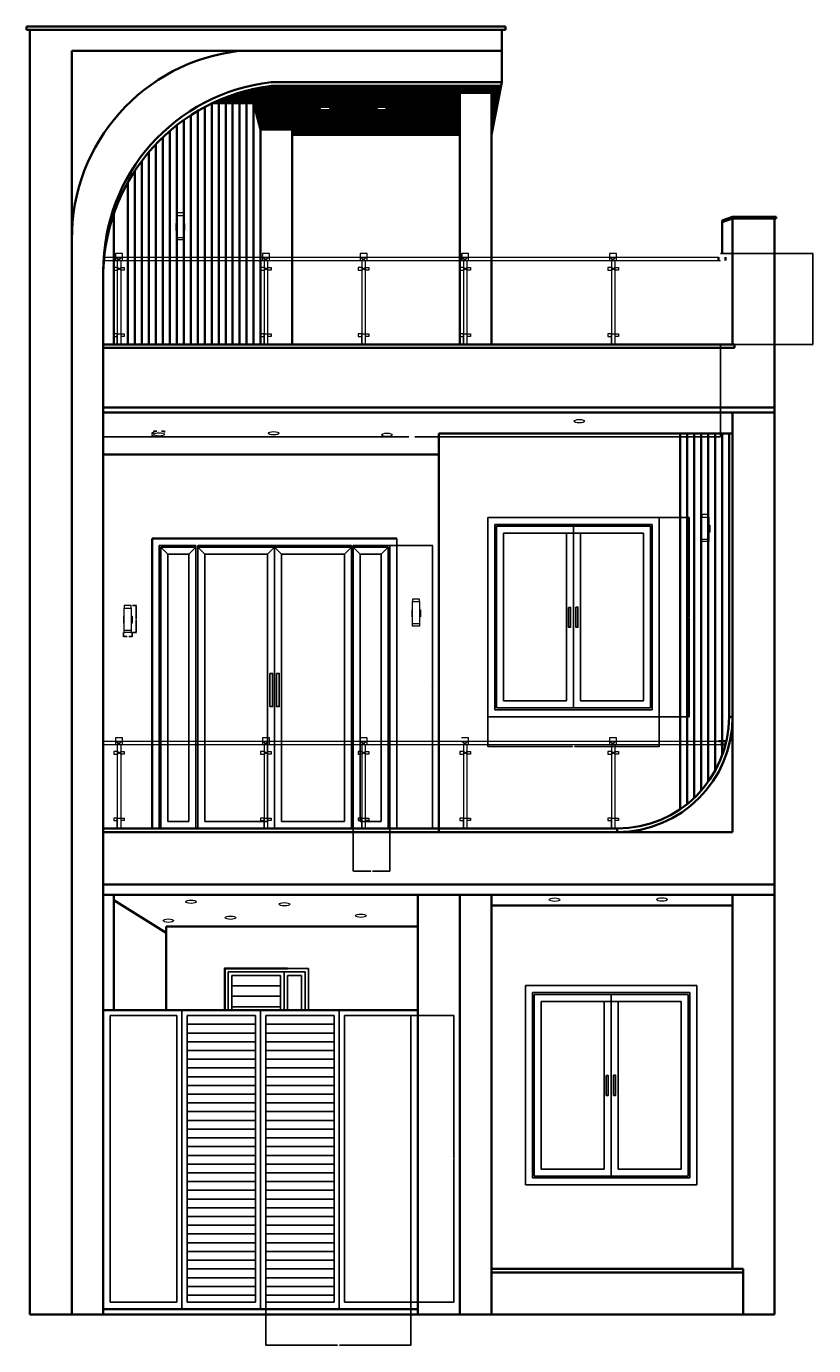
# Model space of a CAD drawing. Units: inches. Extents: x 2700 to 3150, y 1021 to 1776.
import ezdxf

# ---------------------------------------------------------------- set-up
doc = ezdxf.new("R2010")
doc.units = ezdxf.units.IN
doc.header["$MEASUREMENT"] = 0
for name, color, linetype, lineweight in [('A-ANNO-DIMS', 2, 'Continuous', 18), ('A-DOOR', 3, 'Continuous', 25), ('A-ELEV', 7, 'Continuous', 35), ('A-ELEV-CONS', 8, 'Continuous', 13), ('A-FLOR-HRAL', 6, 'Continuous', 18), ('A-GLAZ', 4, 'Continuous', 25), ('E-LITE', 2, 'Continuous', 18)]:
    doc.layers.add(name, color=color, linetype=linetype, lineweight=lineweight)
doc.styles.get("Standard").update_dxf_attribs({"font": 'arial.ttf'})
doc.dimstyles.get("Standard").update_dxf_attribs({"dimtxt": 0.18, "dimasz": 0.18, "dimexe": 0.18, "dimexo": 0.0625, "dimgap": 0.09, "dimtad": 0, "dimtih": 1, "dimtoh": 1, "dimdec": 1, "dimzin": 0, "dimdsep": 46, "dimlunit": 3, "dimtxsty": 'Standard', "dimcen": 0.09, "dimadec": 0, "dimazin": 0, "dimtfac": 1, "dimtdec": 1, "dimtofl": 0, "dimtmove": 0, "dimatfit": 3, "dimfxl": 1, "dimtolj": 1, "dimtzin": 0, "dimarcsym": 0})

# ---------------------------------------------------------------- blocks, each defined once
blk = doc.blocks.new('g')
for p, q in [((2754.61, 1646.14), (2750.61, 1646.14)), ((2750.61, 1646.14), (2750.61, 1642.14)), ((2754.61, 1642.14), (2754.61, 1646.14)), ((2838.61, 1646.14), (2834.61, 1646.14)), ((2834.61, 1646.14), (2834.61, 1642.14)), ((2838.61, 1642.14), (2838.61, 1646.14)), ((2894.49, 1646.14), (2890.49, 1646.14)), ((2890.49, 1646.14), (2890.49, 1642.14)), ((2894.49, 1642.14), (2894.49, 1646.14)), ((2952.61, 1646.14), (2948.61, 1646.14)), ((2952.61, 1642.14), (2952.61, 1646.14)), ((3037.26, 1646.14), (3033.26, 1646.14)), ((3033.26, 1646.14), (3033.26, 1642.14)), ((3037.26, 1642.14), (3037.26, 1646.14)), ((2743.61, 1644.14), (3095.61, 1644.14)), ((2743.61, 1642.14), (3096.61, 1642.14)), ((2751.61, 1638.14), (2749.61, 1638.14)), ((2749.61, 1638.14), (2749.61, 1636.64)), ((2750.61, 1644.14), (2753.61, 1642.14)), ((2750.61, 1642.14), (2751.61, 1642.14)), ((2754.61, 1644.14), (2751.61, 1642.14)), ((2751.61, 1642.14), (2751.61, 1594.14)), ((2751.61, 1636.64), (2753.61, 1638.14)), ((2753.61, 1636.64), (2751.61, 1638.14)), ((2753.61, 1642.14), (2754.61, 1642.14)), ((2753.61, 1642.14), (2753.61, 1594.14)), ((2753.61, 1642.14), (2753.61, 1638.14)), ((2753.61, 1638.14), (2755.61, 1638.14)), ((2755.61, 1638.14), (2755.61, 1636.64)), ((2835.61, 1638.14), (2833.61, 1638.14)), ((2833.61, 1638.14), (2833.61, 1636.64)), ((2834.61, 1644.14), (2837.61, 1642.14)), ((2834.61, 1642.14), (2835.61, 1642.14)), ((2838.61, 1644.14), (2835.61, 1642.14)), ((2835.61, 1642.14), (2835.61, 1594.14)), ((2835.61, 1636.64), (2837.61, 1638.14)), ((2837.61, 1636.64), (2835.61, 1638.14)), ((2837.61, 1642.14), (2838.61, 1642.14)), ((2837.61, 1642.14), (2837.61, 1594.14)), ((2837.61, 1642.14), (2837.61, 1638.14)), ((2837.61, 1638.14), (2839.61, 1638.14)), ((2839.61, 1638.14), (2839.61, 1636.64)), ((2891.49, 1638.14), (2889.49, 1638.14)), ((2889.49, 1638.14), (2889.49, 1636.64)), ((2890.49, 1644.14), (2893.49, 1642.14)), ((2890.49, 1642.14), (2891.49, 1642.14)), ((2894.49, 1644.14), (2891.49, 1642.14)), ((2891.49, 1642.14), (2891.49, 1594.14)), ((2891.49, 1636.64), (2893.49, 1638.14)), ((2893.49, 1636.64), (2891.49, 1638.14)), ((2893.49, 1642.14), (2894.49, 1642.14)), ((2893.49, 1642.14), (2893.49, 1594.14)), ((2893.49, 1642.14), (2893.49, 1638.14)), ((2893.49, 1638.14), (2895.49, 1638.14)), ((2895.49, 1638.14), (2895.49, 1636.64)), ((2949.61, 1638.14), (2947.61, 1638.14)), ((2947.61, 1638.14), (2947.61, 1636.64)), ((2948.61, 1644.14), (2951.61, 1642.14)), ((2948.61, 1642.14), (2949.61, 1642.14)), ((2952.61, 1644.14), (2949.61, 1642.14)), ((2949.61, 1642.14), (2949.61, 1594.14)), ((2949.61, 1636.64), (2951.61, 1638.14)), ((2951.61, 1636.64), (2949.61, 1638.14)), ((2951.61, 1642.14), (2952.61, 1642.14)), ((2951.61, 1642.14), (2951.61, 1594.14)), ((2951.61, 1642.14), (2951.61, 1638.14)), ((2951.61, 1638.14), (2953.61, 1638.14)), ((2953.61, 1638.14), (2953.61, 1636.64)), ((3034.26, 1638.14), (3032.26, 1638.14)), ((3032.26, 1638.14), (3032.26, 1636.64)), ((3033.26, 1644.14), (3036.26, 1642.14)), ((3033.26, 1642.14), (3034.26, 1642.14)), ((3037.26, 1644.14), (3034.26, 1642.14)), ((3034.26, 1642.14), (3034.26, 1594.14)), ((3034.26, 1636.64), (3036.26, 1638.14)), ((3036.26, 1636.64), (3034.26, 1638.14)), ((3036.26, 1642.14), (3037.26, 1642.14)), ((3036.26, 1642.14), (3036.26, 1594.14)), ((3036.26, 1642.14), (3036.26, 1638.14)), ((3036.26, 1638.14), (3038.26, 1638.14)), ((3038.26, 1638.14), (3038.26, 1636.64)), ((2749.61, 1636.64), (2751.61, 1636.64)), ((2755.61, 1636.64), (2753.61, 1636.64)), ((2833.61, 1636.64), (2835.61, 1636.64)), ((2839.61, 1636.64), (2837.61, 1636.64)), ((2889.49, 1636.64), (2891.49, 1636.64)), ((2895.49, 1636.64), (2893.49, 1636.64)), ((2947.61, 1636.64), (2949.61, 1636.64)), ((2953.61, 1636.64), (2951.61, 1636.64)), ((3032.26, 1636.64), (3034.26, 1636.64)), ((3038.26, 1636.64), (3036.26, 1636.64)), ((2751.61, 1600.16), (2749.61, 1600.16)), ((2749.61, 1600.16), (2749.61, 1598.66)), ((2749.61, 1598.66), (2751.61, 1598.66)), ((2751.61, 1594.14), (2751.61, 1600.16)), ((2751.61, 1600.16), (2753.61, 1600.16)), ((2753.61, 1600.16), (2755.61, 1600.16)), ((2755.61, 1598.66), (2753.61, 1598.66)), ((2755.61, 1600.16), (2755.61, 1598.66)), ((2835.61, 1600.16), (2833.61, 1600.16)), ((2833.61, 1600.16), (2833.61, 1598.66)), ((2833.61, 1598.66), (2835.61, 1598.66)), ((2835.61, 1594.14), (2835.61, 1600.16)), ((2835.61, 1600.16), (2837.61, 1600.16)), ((2837.61, 1600.16), (2839.61, 1600.16)), ((2839.61, 1598.66), (2837.61, 1598.66)), ((2839.61, 1600.16), (2839.61, 1598.66)), ((2891.49, 1600.16), (2889.49, 1600.16)), ((2889.49, 1600.16), (2889.49, 1598.66)), ((2889.49, 1598.66), (2891.49, 1598.66)), ((2891.49, 1594.14), (2891.49, 1600.16)), ((2891.49, 1600.16), (2893.49, 1600.16)), ((2893.49, 1600.16), (2895.49, 1600.16)), ((2895.49, 1598.66), (2893.49, 1598.66)), ((2895.49, 1600.16), (2895.49, 1598.66)), ((2949.61, 1600.16), (2947.61, 1600.16)), ((2947.61, 1600.16), (2947.61, 1598.66)), ((2947.61, 1598.66), (2949.61, 1598.66)), ((2949.61, 1594.14), (2949.61, 1600.16)), ((2949.61, 1600.16), (2951.61, 1600.16)), ((2951.61, 1600.16), (2953.61, 1600.16)), ((2953.61, 1598.66), (2951.61, 1598.66)), ((2953.61, 1600.16), (2953.61, 1598.66)), ((3034.26, 1600.16), (3032.26, 1600.16)), ((3032.26, 1600.16), (3032.26, 1598.66)), ((3032.26, 1598.66), (3034.26, 1598.66)), ((3034.26, 1594.14), (3034.26, 1600.16)), ((3034.26, 1600.16), (3036.26, 1600.16)), ((3036.26, 1600.16), (3038.26, 1600.16)), ((3038.26, 1598.66), (3036.26, 1598.66)), ((3038.26, 1600.16), (3038.26, 1598.66))]:
    blk.add_line(p, q)
blk = doc.blocks.new('l')
for p, q in [((3090.07, 1496.8), (3086.07, 1496.8)), ((3086.07, 1496.8), (3086.07, 1495.38)), ((3086.07, 1495.38), (3090.07, 1495.38)), ((3086.07, 1481.35), (3086.07, 1495.38)), ((3090.07, 1495.38), (3090.07, 1496.8)), ((3090.07, 1495.38), (3090.07, 1481.35)), ((3086.07, 1490.73), (3085.61, 1490.73)), ((3085.61, 1490.73), (3085.61, 1486.73)), ((3090.07, 1490.73), (3090.61, 1490.73)), ((3090.61, 1490.73), (3090.61, 1486.73)), ((3085.61, 1486.73), (3086.07, 1486.73)), ((3086.07, 1482.78), (3090.07, 1482.78)), ((3090.07, 1481.35), (3086.07, 1481.35)), ((3090.61, 1486.73), (3090.07, 1486.73))]:
    blk.add_line(p, q)
blk = doc.blocks.new('WIN-DOUBLE')
for p, q in [((2963.61, 1495.14), (2963.61, 1381.14)), ((2963.61, 1495.14), (3061.61, 1495.14)), ((3061.61, 1495.14), (3061.61, 1381.14)), ((2967.61, 1491.14), (2967.61, 1385.14)), ((2967.61, 1491.14), (3057.61, 1491.14)), ((2968.61, 1490.14), (2968.61, 1386.14)), ((2968.61, 1490.14), (3056.61, 1490.14)), ((3012.61, 1490.14), (3012.61, 1386.14)), ((3056.61, 1490.14), (3056.61, 1386.14)), ((3057.61, 1491.14), (3057.61, 1385.14)), ((2972.61, 1486.14), (3052.61, 1486.14)), ((2972.61, 1486.14), (2972.61, 1390.14)), ((3008.61, 1486.14), (3008.61, 1390.14)), ((3016.61, 1486.14), (3016.61, 1390.14)), ((3052.61, 1486.14), (3052.61, 1390.14)), ((2972.61, 1390.14), (3008.61, 1390.14)), ((3016.61, 1390.14), (3052.61, 1390.14)), ((2967.61, 1385.14), (3057.61, 1385.14)), ((2968.61, 1386.14), (3056.61, 1386.14)), ((2963.61, 1381.14), (3061.61, 1381.14))]:
    blk.add_line(p, q)
for points in [[(3009.78, 1443.68), (3010.92, 1443.68), (3010.92, 1432.35), (3009.78, 1432.35)], [(3013.96, 1443.85), (3015.09, 1443.85), (3015.09, 1432.33), (3013.96, 1432.33)]]:
    blk.add_lwpolyline(points, close=True)
blk = doc.blocks.new('DOOR-SIDELIGHT')
for p, q in [((2886.61, 1317.14), (2886.61, 1479.14)), ((2886.61, 1479.14), (2907.61, 1479.14)), ((2886.61, 1478.14), (2906.61, 1478.14)), ((2890.61, 1474.14), (2886.61, 1478.14)), ((2890.61, 1321.14), (2890.61, 1474.14)), ((2890.61, 1474.14), (2902.61, 1474.14)), ((2902.61, 1474.14), (2906.61, 1478.14)), ((2902.61, 1321.14), (2902.61, 1474.14)), ((2906.61, 1317.14), (2906.61, 1478.14)), ((2907.61, 1317.14), (2907.61, 1479.14)), ((2890.61, 1321.14), (2902.61, 1321.14))]:
    blk.add_line(p, q)
blk = doc.blocks.new('GATE-SIDE-PANEL')
for p, q in [((2836.61, 1210.14), (2836.61, 1046.14)), ((2875.61, 1210.14), (2836.61, 1210.14)), ((2875.61, 1210.14), (2875.61, 1046.14)), ((2881.61, 1210.14), (2881.61, 1046.14)), ((2919.61, 1210.14), (2881.61, 1210.14)), ((2919.61, 1210.14), (2919.61, 1046.14)), ((2836.61, 1046.14), (2875.61, 1046.14)), ((2881.61, 1046.14), (2919.61, 1046.14))]:
    blk.add_line(p, q)
blk = doc.blocks.new('LIGHT-COVE')
blk.add_ellipse((2870.52, 1729.14), major_axis=(-3.07, 0), ratio=0.316207)
blk = doc.blocks.new('*D7')
at = {"layer": 'A-ANNO-DIMS', "color": 0, "lineweight": -2, "transparency": 16777216}
for p, q in [((3061.67, 1495.14), (3078.89, 1495.14)), ((3078.71, 1494.96), (3078.71, 1438.32)), ((3078.71, 1381.32), (3078.71, 1437.96)), ((3061.67, 1381.14), (3078.89, 1381.14))]:
    blk.add_line(p, q, dxfattribs=at)
at = {"layer": 'A-ANNO-DIMS', "color": 0, "transparency": 16777216}
for points in [[(3078.68, 1494.96), (3078.74, 1494.96), (3078.71, 1495.14)], [(3078.68, 1381.32), (3078.74, 1381.32), (3078.71, 1381.14)]]:
    blk.add_solid(points, dxfattribs=at)
at = {"layer": 'Defpoints', "color": 0, "transparency": 16777216}
for p in [(3061.61, 1495.14), (3078.71, 1495.14), (3061.61, 1381.14)]:
    blk.add_point(p, dxfattribs=at)
at = {"layer": 'A-ANNO-DIMS', "color": 0, "transparency": 16777216, "insert": (3078.71, 1438.14), "char_height": 0.18, "attachment_point": 5}
blk.add_mtext('\\A1;WINDOW 114 TYP.', dxfattribs=at)
blk = doc.blocks.new('*D8')
at = {"layer": 'A-ANNO-DIMS', "color": 0, "lineweight": -2, "transparency": 16777216}
for p, q in [((2963.61, 1381.08), (2963.61, 1363.86)), ((3061.61, 1381.08), (3061.61, 1363.86)), ((2963.79, 1364.04), (3012.08, 1364.04)), ((3061.43, 1364.04), (3013.14, 1364.04))]:
    blk.add_line(p, q, dxfattribs=at)
at = {"layer": 'A-ANNO-DIMS', "color": 0, "transparency": 16777216}
for points in [[(2963.79, 1364.07), (2963.79, 1364.01), (2963.61, 1364.04)], [(3061.43, 1364.07), (3061.43, 1364.01), (3061.61, 1364.04)]]:
    blk.add_solid(points, dxfattribs=at)
at = {"layer": 'Defpoints', "color": 0, "transparency": 16777216}
for p in [(2963.61, 1381.14), (3061.61, 1381.14), (3061.61, 1364.04)]:
    blk.add_point(p, dxfattribs=at)
at = {"layer": 'A-ANNO-DIMS', "color": 0, "transparency": 16777216, "insert": (3012.61, 1364.04), "char_height": 0.18, "attachment_point": 5}
blk.add_mtext('\\A1;98 TYP.', dxfattribs=at)
blk = doc.blocks.new('*D9')
at = {"layer": 'A-ANNO-DIMS', "color": 0, "lineweight": -2, "transparency": 16777216}
for p, q in [((2907.67, 1479.14), (2932.09, 1479.14)), ((2931.91, 1478.96), (2931.91, 1398.32)), ((2931.91, 1317.32), (2931.91, 1397.96)), ((2907.67, 1317.14), (2932.09, 1317.14))]:
    blk.add_line(p, q, dxfattribs=at)
at = {"layer": 'A-ANNO-DIMS', "color": 0, "transparency": 16777216}
for points in [[(2931.88, 1478.96), (2931.94, 1478.96), (2931.91, 1479.14)], [(2931.88, 1317.32), (2931.94, 1317.32), (2931.91, 1317.14)]]:
    blk.add_solid(points, dxfattribs=at)
at = {"layer": 'Defpoints', "color": 0, "transparency": 16777216}
for p in [(2907.61, 1479.14), (2931.91, 1479.14), (2907.61, 1317.14)]:
    blk.add_point(p, dxfattribs=at)
at = {"layer": 'A-ANNO-DIMS', "color": 0, "transparency": 16777216, "insert": (2931.91, 1398.14), "char_height": 0.18, "attachment_point": 5}
blk.add_mtext('\\A1;DOOR SIDELIGHT 162 TYP.', dxfattribs=at)
blk = doc.blocks.new('*D10')
at = {"layer": 'A-ANNO-DIMS', "color": 0, "lineweight": -2, "transparency": 16777216}
for p, q in [((2886.61, 1317.08), (2886.61, 1292.66)), ((2907.61, 1317.08), (2907.61, 1292.66)), ((2886.79, 1292.84), (2896.58, 1292.84)), ((2907.43, 1292.84), (2897.64, 1292.84))]:
    blk.add_line(p, q, dxfattribs=at)
at = {"layer": 'A-ANNO-DIMS', "color": 0, "transparency": 16777216}
for points in [[(2886.79, 1292.87), (2886.79, 1292.81), (2886.61, 1292.84)], [(2907.43, 1292.87), (2907.43, 1292.81), (2907.61, 1292.84)]]:
    blk.add_solid(points, dxfattribs=at)
at = {"layer": 'Defpoints', "color": 0, "transparency": 16777216}
for p in [(2886.61, 1317.14), (2907.61, 1317.14), (2907.61, 1292.84)]:
    blk.add_point(p, dxfattribs=at)
at = {"layer": 'A-ANNO-DIMS', "color": 0, "transparency": 16777216, "insert": (2897.11, 1292.84), "char_height": 0.18, "attachment_point": 5}
blk.add_mtext('\\A1;21 TYP.', dxfattribs=at)
blk = doc.blocks.new('*D11')
at = {"layer": 'A-ANNO-DIMS', "color": 0, "lineweight": -2, "transparency": 16777216}
for p, q in [((2919.67, 1210.14), (2944.39, 1210.14)), ((2944.21, 1209.96), (2944.21, 1128.32)), ((2944.21, 1046.32), (2944.21, 1127.96)), ((2919.67, 1046.14), (2944.39, 1046.14))]:
    blk.add_line(p, q, dxfattribs=at)
at = {"layer": 'A-ANNO-DIMS', "color": 0, "transparency": 16777216}
for points in [[(2944.18, 1209.96), (2944.24, 1209.96), (2944.21, 1210.14)], [(2944.18, 1046.32), (2944.24, 1046.32), (2944.21, 1046.14)]]:
    blk.add_solid(points, dxfattribs=at)
at = {"layer": 'Defpoints', "color": 0, "transparency": 16777216}
for p in [(2919.61, 1210.14), (2944.21, 1210.14), (2919.61, 1046.14)]:
    blk.add_point(p, dxfattribs=at)
at = {"layer": 'A-ANNO-DIMS', "color": 0, "transparency": 16777216, "insert": (2944.21, 1128.14), "char_height": 0.18, "attachment_point": 5}
blk.add_mtext('\\A1;GATE SIDE PANEL 164 TYP.', dxfattribs=at)
blk = doc.blocks.new('*D12')
at = {"layer": 'A-ANNO-DIMS', "color": 0, "lineweight": -2, "transparency": 16777216}
for p, q in [((2836.61, 1046.08), (2836.61, 1021.36)), ((2919.61, 1046.08), (2919.61, 1021.36)), ((2836.79, 1021.54), (2877.58, 1021.54)), ((2919.43, 1021.54), (2878.64, 1021.54))]:
    blk.add_line(p, q, dxfattribs=at)
at = {"layer": 'A-ANNO-DIMS', "color": 0, "transparency": 16777216}
for points in [[(2836.79, 1021.57), (2836.79, 1021.51), (2836.61, 1021.54)], [(2919.43, 1021.57), (2919.43, 1021.51), (2919.61, 1021.54)]]:
    blk.add_solid(points, dxfattribs=at)
at = {"layer": 'Defpoints', "color": 0, "transparency": 16777216}
for p in [(2836.61, 1046.14), (2919.61, 1046.14), (2919.61, 1021.54)]:
    blk.add_point(p, dxfattribs=at)
at = {"layer": 'A-ANNO-DIMS', "color": 0, "transparency": 16777216, "insert": (2878.11, 1021.54), "char_height": 0.18, "attachment_point": 5}
blk.add_mtext('\\A1;83 TYP.', dxfattribs=at)
blk = doc.blocks.new('*D13')
at = {"layer": 'A-ANNO-DIMS', "color": 0, "lineweight": -2, "transparency": 16777216}
for p, q in [((2743.61, 1594.08), (2743.61, 1541.01)), ((3096.61, 1594.08), (3096.61, 1541.01)), ((2743.79, 1541.19), (2918.34, 1541.19)), ((3096.43, 1541.19), (2921.88, 1541.19))]:
    blk.add_line(p, q, dxfattribs=at)
at = {"layer": 'A-ANNO-DIMS', "color": 0, "transparency": 16777216}
for points in [[(2743.79, 1541.22), (2743.79, 1541.16), (2743.61, 1541.19)], [(3096.43, 1541.22), (3096.43, 1541.16), (3096.61, 1541.19)]]:
    blk.add_solid(points, dxfattribs=at)
at = {"layer": 'Defpoints', "color": 0, "transparency": 16777216}
for p in [(2743.61, 1594.14), (3096.61, 1594.14), (3096.61, 1541.19)]:
    blk.add_point(p, dxfattribs=at)
at = {"layer": 'A-ANNO-DIMS', "color": 0, "transparency": 16777216, "insert": (2920.11, 1541.19), "char_height": 0.18, "attachment_point": 5}
blk.add_mtext('\\A1;BALCONY RAILING 353 TYP.', dxfattribs=at)
blk = doc.blocks.new('*D14')
at = {"layer": 'A-ANNO-DIMS', "color": 0, "lineweight": -2, "transparency": 16777216}
for p, q in [((3096.67, 1646.14), (3149.74, 1646.14)), ((3149.56, 1645.96), (3149.56, 1620.32)), ((3149.56, 1594.32), (3149.56, 1619.96)), ((3096.67, 1594.14), (3149.74, 1594.14))]:
    blk.add_line(p, q, dxfattribs=at)
at = {"layer": 'A-ANNO-DIMS', "color": 0, "transparency": 16777216}
for points in [[(3149.53, 1645.96), (3149.59, 1645.96), (3149.56, 1646.14)], [(3149.53, 1594.32), (3149.59, 1594.32), (3149.56, 1594.14)]]:
    blk.add_solid(points, dxfattribs=at)
at = {"layer": 'Defpoints', "color": 0, "transparency": 16777216}
for p in [(3096.61, 1646.14), (3149.56, 1646.14), (3096.61, 1594.14)]:
    blk.add_point(p, dxfattribs=at)
at = {"layer": 'A-ANNO-DIMS', "color": 0, "transparency": 16777216, "insert": (3149.56, 1620.14), "char_height": 0.18, "attachment_point": 5}
blk.add_mtext('\\A1;52 TYP.', dxfattribs=at)
blk = doc.blocks.new('*D15')
at = {"layer": 'A-ANNO-DIMS', "color": 0, "lineweight": -2, "transparency": 16777216}
for p, q in [((2772.49, 1543.72), (2772.49, 1544.75)), ((2772.67, 1544.57), (2774.3, 1544.57)), ((2778.45, 1544.57), (2776.81, 1544.57)), ((2778.63, 1543.72), (2778.63, 1544.75))]:
    blk.add_line(p, q, dxfattribs=at)
at = {"layer": 'A-ANNO-DIMS', "color": 0, "transparency": 16777216}
for points in [[(2772.67, 1544.6), (2772.67, 1544.54), (2772.49, 1544.57)], [(2778.45, 1544.6), (2778.45, 1544.54), (2778.63, 1544.57)]]:
    blk.add_solid(points, dxfattribs=at)
at = {"layer": 'Defpoints', "color": 0, "transparency": 16777216}
for p in [(2772.49, 1544.57), (2772.49, 1543.65), (2778.63, 1543.65)]:
    blk.add_point(p, dxfattribs=at)
at = {"layer": 'A-ANNO-DIMS', "color": 0, "transparency": 16777216, "insert": (2775.56, 1544.57), "char_height": 0.18, "attachment_point": 5}
blk.add_mtext('\\A1;DOWNLIGHT 6 TYP.', dxfattribs=at)
blk = doc.blocks.new('*D16')
at = {"layer": 'A-ANNO-DIMS', "color": 0, "lineweight": -2, "transparency": 16777216}
for p, q in [((2772.43, 1543.65), (2771.39, 1543.65)), ((2772.43, 1541.71), (2771.39, 1541.71)), ((2771.57, 1543.47), (2771.57, 1542.86)), ((2771.57, 1541.89), (2771.57, 1542.5))]:
    blk.add_line(p, q, dxfattribs=at)
at = {"layer": 'A-ANNO-DIMS', "color": 0, "transparency": 16777216}
for points in [[(2771.54, 1543.47), (2771.6, 1543.47), (2771.57, 1543.65)], [(2771.54, 1541.89), (2771.6, 1541.89), (2771.57, 1541.71)]]:
    blk.add_solid(points, dxfattribs=at)
at = {"layer": 'Defpoints', "color": 0, "transparency": 16777216}
for p in [(2771.57, 1541.71), (2772.49, 1543.65), (2772.49, 1541.71)]:
    blk.add_point(p, dxfattribs=at)
at = {"layer": 'A-ANNO-DIMS', "color": 0, "transparency": 16777216, "insert": (2771.57, 1542.68), "char_height": 0.18, "attachment_point": 5}
blk.add_mtext('\\A1;2 TYP.', dxfattribs=at)
blk = doc.blocks.new('*D17')
at = {"layer": 'A-ANNO-DIMS', "color": 0, "lineweight": -2, "transparency": 16777216}
for p, q in [((2760.23, 1444.73), (2762.66, 1444.73)), ((2762.48, 1444.55), (2762.48, 1437.19)), ((2762.48, 1429.47), (2762.48, 1436.83)), ((2760.23, 1429.29), (2762.66, 1429.29))]:
    blk.add_line(p, q, dxfattribs=at)
at = {"layer": 'A-ANNO-DIMS', "color": 0, "transparency": 16777216}
for points in [[(2762.45, 1444.55), (2762.51, 1444.55), (2762.48, 1444.73)], [(2762.45, 1429.47), (2762.51, 1429.47), (2762.48, 1429.29)]]:
    blk.add_solid(points, dxfattribs=at)
at = {"layer": 'Defpoints', "color": 0, "transparency": 16777216}
for p in [(2760.16, 1444.73), (2762.48, 1444.73), (2760.16, 1429.29)]:
    blk.add_point(p, dxfattribs=at)
at = {"layer": 'A-ANNO-DIMS', "color": 0, "transparency": 16777216, "insert": (2762.48, 1437.01), "char_height": 0.18, "attachment_point": 5}
blk.add_mtext('\\A1;WALL LIGHT 15 TYP.', dxfattribs=at)
blk = doc.blocks.new('*D18')
at = {"layer": 'A-ANNO-DIMS', "color": 0, "lineweight": -2, "transparency": 16777216}
for p, q in [((2755.16, 1429.23), (2755.16, 1426.79)), ((2755.34, 1426.97), (2757.2, 1426.97)), ((2759.98, 1426.97), (2758.12, 1426.97)), ((2760.16, 1429.23), (2760.16, 1426.79))]:
    blk.add_line(p, q, dxfattribs=at)
at = {"layer": 'A-ANNO-DIMS', "color": 0, "transparency": 16777216}
for points in [[(2755.34, 1427), (2755.34, 1426.94), (2755.16, 1426.97)], [(2759.98, 1427), (2759.98, 1426.94), (2760.16, 1426.97)]]:
    blk.add_solid(points, dxfattribs=at)
at = {"layer": 'Defpoints', "color": 0, "transparency": 16777216}
for p in [(2755.16, 1429.29), (2760.16, 1429.29), (2760.16, 1426.97)]:
    blk.add_point(p, dxfattribs=at)
at = {"layer": 'A-ANNO-DIMS', "color": 0, "transparency": 16777216, "insert": (2757.66, 1426.97), "char_height": 0.18, "attachment_point": 5}
blk.add_mtext('\\A1;5 TYP.', dxfattribs=at)

msp = doc.modelspace()

# ---------------------------------------------------------------- linework, layer by layer
at = {"layer": 'A-DOOR'}
for p, q in [((2911.61, 1317.14), (2911.61, 1483.14)), ((2797.61, 1317.14), (2797.61, 1479.14)), ((2797.61, 1479.14), (2885.61, 1479.14)), ((2797.61, 1478.14), (2885.61, 1478.14)), ((2801.61, 1474.14), (2797.61, 1478.14)), ((2801.61, 1321.14), (2801.61, 1474.14)), ((2801.61, 1474.14), (2837.61, 1474.14)), ((2841.61, 1478.14), (2837.61, 1474.14)), ((2837.61, 1321.14), (2837.61, 1474.14)), ((2841.61, 1317.14), (2841.61, 1478.14)), ((2845.61, 1474.14), (2841.61, 1478.14)), ((2845.61, 1321.14), (2845.61, 1474.14)), ((2845.61, 1474.14), (2881.61, 1474.14)), ((2881.61, 1474.14), (2885.61, 1478.14)), ((2881.61, 1321.14), (2881.61, 1474.14)), ((2885.61, 1317.14), (2885.61, 1479.14)), ((2801.61, 1321.14), (2837.61, 1321.14)), ((2845.61, 1321.14), (2881.61, 1321.14)), ((2788.61, 1213.14), (2788.61, 1042.14)), ((2833.61, 1213.14), (2833.61, 1042.14)), ((2878.61, 1213.14), (2878.61, 1042.14)), ((2830.61, 1205.14), (2791.61, 1205.14)), ((2875.61, 1205.14), (2836.61, 1205.14)), ((2830.61, 1200.14), (2791.61, 1200.14)), ((2830.61, 1195.14), (2791.61, 1195.14)), ((2875.61, 1200.14), (2836.61, 1200.14)), ((2875.61, 1195.14), (2836.61, 1195.14)), ((2830.61, 1190.14), (2791.61, 1190.14)), ((2875.61, 1190.14), (2836.61, 1190.14)), ((2830.61, 1185.14), (2791.61, 1185.14)), ((2830.61, 1180.14), (2791.61, 1180.14)), ((2875.61, 1185.14), (2836.61, 1185.14)), ((2875.61, 1180.14), (2836.61, 1180.14)), ((2830.61, 1175.14), (2791.61, 1175.14)), ((2830.61, 1170.14), (2791.61, 1170.14)), ((2875.61, 1175.14), (2836.61, 1175.14)), ((2875.61, 1170.14), (2836.61, 1170.14)), ((2830.61, 1165.14), (2791.61, 1165.14)), ((2875.61, 1165.14), (2836.61, 1165.14)), ((2830.61, 1160.14), (2791.61, 1160.14)), ((2830.61, 1155.14), (2791.61, 1155.14)), ((2875.61, 1160.14), (2836.61, 1160.14)), ((2875.61, 1155.14), (2836.61, 1155.14)), ((2830.61, 1150.14), (2791.61, 1150.14)), ((2875.61, 1150.14), (2836.61, 1150.14)), ((2830.61, 1145.14), (2791.61, 1145.14)), ((2830.61, 1140.14), (2791.61, 1140.14)), ((2875.61, 1145.14), (2836.61, 1145.14)), ((2875.61, 1140.14), (2836.61, 1140.14)), ((2830.61, 1135.14), (2791.61, 1135.14)), ((2875.61, 1135.14), (2836.61, 1135.14)), ((2830.61, 1130.14), (2791.61, 1130.14)), ((2830.61, 1125.14), (2791.61, 1125.14)), ((2875.61, 1130.14), (2836.61, 1130.14)), ((2875.61, 1125.14), (2836.61, 1125.14)), ((2830.61, 1120.14), (2791.61, 1120.14)), ((2875.61, 1120.14), (2836.61, 1120.14)), ((2830.61, 1115.14), (2791.61, 1115.14)), ((2830.61, 1110.14), (2791.61, 1110.14)), ((2875.61, 1115.14), (2836.61, 1115.14)), ((2875.61, 1110.14), (2836.61, 1110.14)), ((2830.61, 1105.14), (2791.61, 1105.14)), ((2875.61, 1105.14), (2836.61, 1105.14)), ((2830.61, 1100.14), (2791.61, 1100.14)), ((2830.61, 1095.14), (2791.61, 1095.14)), ((2875.61, 1100.14), (2836.61, 1100.14)), ((2875.61, 1095.14), (2836.61, 1095.14)), ((2830.61, 1090.14), (2791.61, 1090.14)), ((2875.61, 1090.14), (2836.61, 1090.14)), ((2830.61, 1085.14), (2791.61, 1085.14)), ((2830.61, 1080.14), (2791.61, 1080.14)), ((2875.61, 1085.14), (2836.61, 1085.14)), ((2875.61, 1080.14), (2836.61, 1080.14)), ((2830.61, 1075.14), (2791.61, 1075.14)), ((2875.61, 1075.14), (2836.61, 1075.14)), ((2830.61, 1070.14), (2791.61, 1070.14)), ((2830.61, 1065.14), (2791.61, 1065.14)), ((2875.61, 1070.14), (2836.61, 1070.14)), ((2875.61, 1065.14), (2836.61, 1065.14)), ((2830.61, 1060.14), (2791.61, 1060.14)), ((2875.61, 1060.14), (2836.61, 1060.14)), ((2830.61, 1055.14), (2791.61, 1055.14)), ((2830.61, 1050.14), (2791.61, 1050.14)), ((2875.61, 1055.14), (2836.61, 1055.14)), ((2875.61, 1050.14), (2836.61, 1050.14))]:
    msp.add_line(p, q, dxfattribs=at)
for points in [[(2838.88, 1405.9), (2840.47, 1405.9), (2840.47, 1386.9), (2838.88, 1386.9)], [(2842.67, 1405.9), (2844.26, 1405.9), (2844.26, 1386.9), (2842.67, 1386.9)]]:
    msp.add_lwpolyline(points, close=True, dxfattribs=at)
at = {"layer": 'A-ELEV'}
for p, q in [((2701.61, 1776.14), (2699.61, 1776.14)), ((2699.61, 1776.14), (2699.61, 1774.14)), ((2699.61, 1774.14), (2701.61, 1774.14)), ((2701.61, 1776.14), (2971.61, 1776.14)), ((2701.61, 1039.14), (2701.61, 1774.14)), ((2701.61, 1774.14), (2971.61, 1774.14)), ((2973.61, 1776.14), (2971.61, 1776.14)), ((2971.61, 1744.14), (2971.61, 1774.14)), ((2971.61, 1774.14), (2973.61, 1774.14)), ((2973.61, 1774.14), (2973.61, 1776.14)), ((2725.61, 1039.14), (2725.61, 1762.14)), ((2725.61, 1762.14), (2971.61, 1762.14)), ((2839.61, 1744.14), (2971.61, 1744.14)), ((2971.61, 1744.14), (2965.61, 1714.14)), ((2818.11, 1737.14), (2947.61, 1737.14)), ((2821.19, 1738.14), (2947.61, 1738.14)), ((2824.64, 1739.14), (2970.61, 1739.14)), ((2828.59, 1740.14), (2970.81, 1740.14)), ((2833.35, 1741.14), (2971.01, 1741.14)), ((2839.61, 1742.14), (2971.21, 1742.14)), ((2947.61, 1738.14), (2947.61, 1594.14)), ((2970.41, 1738.14), (2947.61, 1738.14)), ((2965.61, 1738.14), (2965.61, 1594.14)), ((2965.61, 1737.14), (2970.21, 1737.14)), ((2801.61, 1729.97), (2801.61, 1594.14)), ((2805.61, 1732.01), (2805.61, 1594.14)), ((2829.61, 1732.14), (2805.89, 1732.14)), ((2808.02, 1733.14), (2947.61, 1733.14)), ((2809.61, 1732.14), (2809.61, 1594.14)), ((2810.29, 1734.14), (2947.61, 1734.14)), ((2812.7, 1735.14), (2947.61, 1735.14)), ((2813.61, 1732.14), (2813.61, 1594.14)), ((2815.3, 1736.14), (2947.61, 1736.14)), ((2817.61, 1732.14), (2817.61, 1594.14)), ((2821.61, 1732.14), (2821.61, 1594.14)), ((2825.61, 1732.14), (2825.61, 1594.14)), ((2829.61, 1732.14), (2829.61, 1594.14)), ((2829.61, 1732.14), (2947.61, 1732.14)), ((2829.61, 1732.14), (2833.61, 1717.14)), ((2829.87, 1731.14), (2947.61, 1731.14)), ((2830.14, 1730.14), (2947.61, 1730.14)), ((2830.41, 1729.14), (2867.35, 1729.14)), ((2873.49, 1729.14), (2900.06, 1729.14)), ((2905.73, 1729.14), (2947.61, 1729.14)), ((2965.61, 1736.14), (2970.01, 1736.14)), ((2965.61, 1735.14), (2969.81, 1735.14)), ((2965.61, 1734.14), (2969.61, 1734.14)), ((2965.61, 1733.14), (2969.41, 1733.14)), ((2965.61, 1732.14), (2969.21, 1732.14)), ((2965.61, 1731.14), (2969.01, 1731.14)), ((2965.61, 1730.14), (2968.81, 1730.14)), ((2965.61, 1729.14), (2968.61, 1729.14)), ((2789.61, 1722.51), (2789.61, 1594.14)), ((2793.61, 1725.23), (2793.61, 1594.14)), ((2797.61, 1727.71), (2797.61, 1594.14)), ((2830.67, 1728.14), (2947.61, 1728.14)), ((2830.94, 1727.14), (2947.61, 1727.14)), ((2831.21, 1726.14), (2947.61, 1726.14)), ((2831.47, 1725.14), (2947.61, 1725.14)), ((2831.74, 1724.14), (2947.61, 1724.14)), ((2832.01, 1723.14), (2947.61, 1723.14)), ((2832.27, 1722.14), (2947.61, 1722.14)), ((2832.54, 1721.14), (2947.61, 1721.14)), ((2965.61, 1728.14), (2968.41, 1728.14)), ((2965.61, 1727.14), (2968.21, 1727.14)), ((2965.61, 1726.14), (2968.01, 1726.14)), ((2965.61, 1725.14), (2967.81, 1725.14)), ((2965.61, 1724.14), (2967.61, 1724.14)), ((2965.61, 1723.14), (2967.41, 1723.14)), ((2965.61, 1722.14), (2967.21, 1722.14)), ((2965.61, 1721.14), (2967.01, 1721.14)), ((2781.61, 1716.21), (2781.61, 1594.14)), ((2785.61, 1719.51), (2785.61, 1594.14)), ((2832.81, 1720.14), (2947.61, 1720.14)), ((2833.07, 1719.14), (2947.61, 1719.14)), ((2833.34, 1718.14), (2947.61, 1718.14)), ((2833.61, 1717.14), (2833.61, 1594.14)), ((2833.61, 1717.14), (2947.61, 1717.14)), ((2851.61, 1717.14), (2851.61, 1594.14)), ((2851.61, 1716.14), (2947.61, 1716.14)), ((2851.61, 1715.14), (2947.61, 1715.14)), ((2851.61, 1714.14), (2947.61, 1714.14)), ((2965.61, 1720.14), (2966.81, 1720.14)), ((2965.61, 1719.14), (2966.61, 1719.14)), ((2965.61, 1718.14), (2966.41, 1718.14)), ((2965.61, 1717.14), (2966.21, 1717.14)), ((2773.61, 1708.55), (2773.61, 1594.14)), ((2777.61, 1712.57), (2777.61, 1594.14)), ((2765.61, 1699.07), (2765.61, 1594.14)), ((2769.61, 1704.08), (2769.61, 1594.14)), ((2761.61, 1693.37), (2761.61, 1594.14)), ((2757.61, 1686.79), (2757.61, 1594.14)), ((2749.61, 1668.97), (2749.61, 1594.14)), ((3097.61, 1665.14), (3103.61, 1667.14)), ((3103.61, 1666.14), (3097.61, 1664.14)), ((3097.61, 1664.14), (3097.61, 1665.14)), ((3097.61, 1664.14), (3097.61, 1646.14)), ((3103.61, 1667.14), (3103.61, 1594.14)), ((3103.61, 1667.14), (3127.61, 1667.14)), ((3103.61, 1666.14), (3127.61, 1666.14)), ((3127.61, 1667.14), (3128.61, 1667.14)), ((3127.61, 1666.14), (3127.61, 1039.14)), ((3128.61, 1666.14), (3127.61, 1666.14)), ((3128.61, 1667.14), (3128.61, 1666.14)), ((2948.61, 1646.14), (2948.61, 1642.14)), ((3095.61, 1644.14), (3095.61, 1642.14)), ((3099.61, 1644.14), (3099.61, 1642.14)), ((2743.61, 1039.14), (2743.61, 1637.48)), ((2743.61, 1594.14), (3103.61, 1594.14)), ((3103.61, 1594.14), (3104.61, 1594.14)), ((3104.61, 1594.14), (3104.61, 1592.14)), ((2743.61, 1592.14), (3103.61, 1592.14)), ((3104.61, 1592.14), (3103.61, 1592.14)), ((2743.61, 1558.14), (3127.61, 1558.14)), ((2743.61, 1555.14), (3127.61, 1555.14)), ((3103.61, 1555.14), (3103.61, 1315.14)), ((2935.61, 1315.14), (2935.61, 1543.14)), ((2935.61, 1543.14), (3103.61, 1543.14)), ((3073.61, 1543.14), (3073.61, 1328.23)), ((3077.61, 1543.14), (3077.61, 1331.18)), ((3081.61, 1543.14), (3081.61, 1334.66)), ((3085.61, 1543.14), (3085.61, 1338.81)), ((3089.61, 1543.14), (3089.61, 1343.83)), ((3093.61, 1543.14), (3093.61, 1350.16)), ((3097.61, 1543.14), (3097.61, 1358.87)), ((3103.61, 1543.14), (3101.61, 1543.14)), ((3101.61, 1543.14), (3101.61, 1381.14)), ((2743.61, 1531.14), (2935.61, 1531.14)), ((2771.61, 1317.14), (2771.61, 1483.14)), ((2771.61, 1483.14), (2911.61, 1483.14)), ((3103.61, 1381.14), (3101.61, 1381.14)), ((3095.61, 1367.14), (3100.05, 1367.1)), ((3096.61, 1365.14), (3099.58, 1365.15)), ((2743.61, 1317.14), (3037.61, 1317.14)), ((2743.61, 1315.14), (3103.61, 1315.14)), ((3037.61, 1317.14), (3037.61, 1315.14)), ((2743.61, 1285.14), (3127.61, 1285.14)), ((2743.61, 1279.14), (3127.61, 1279.14)), ((2749.61, 1279.14), (2749.61, 1213.14)), ((2749.61, 1276.13), (2779.61, 1257.45)), ((2923.61, 1279.14), (2923.61, 1039.14)), ((2947.61, 1279.14), (2947.61, 1039.14)), ((2947.61, 1279.14), (2947.61, 1039.14)), ((2965.61, 1279.14), (2965.61, 1039.14)), ((3103.61, 1279.14), (3103.61, 1065.14)), ((2965.61, 1273.14), (3103.61, 1273.14)), ((2923.61, 1261.14), (2779.61, 1261.14)), ((2779.61, 1261.14), (2779.61, 1213.14)), ((2923.61, 1213.14), (2743.61, 1213.14)), ((2965.61, 1065.14), (3109.61, 1065.14)), ((3109.61, 1065.14), (3109.61, 1039.14)), ((2965.61, 1063.14), (3109.61, 1063.14)), ((2743.61, 1042.14), (2923.61, 1042.14)), ((2701.61, 1039.14), (3127.61, 1039.14))]:
    msp.add_line(p, q, dxfattribs=at)
msp.add_lwpolyline([(2813.05, 1213.14), (2813.05, 1237.14), (2849.05, 1237.14)], dxfattribs=at)
for centre, radius, start, end in [((2833.61, 1654.81), 108, 96.37827, 180.35466), ((2851.61, 1636.81), 108, 96.37827, 180.35466), ((2853.58, 1633), 110.02, 97.17859, 178.35781), ((3037.61, 1381.14), 66, 270, 0), ((3037.61, 1381.14), 64, 270, 0)]:
    msp.add_arc(centre, radius, start, end, dxfattribs=at)
at = {"layer": 'A-ELEV-CONS'}
for p in [(2788.61, 1213.14), (2833.61, 1213.14), (2878.61, 1213.14)]:
    msp.add_point(p, dxfattribs=at)
at = {"layer": 'A-GLAZ'}
for p, q in [((2817.05, 1213.14), (2817.05, 1233.14)), ((2817.05, 1233.14), (2845.05, 1233.14)), ((2845.05, 1233.14), (2845.05, 1213.14)), ((2847.05, 1235.14), (2859.05, 1235.14)), ((2849.05, 1237.14), (2861.05, 1237.14)), ((2849.05, 1233.14), (2857.05, 1233.14)), ((2857.05, 1233.14), (2857.05, 1213.14)), ((2859.05, 1235.14), (2859.05, 1213.14)), ((2861.05, 1237.14), (2861.05, 1213.14)), ((2817.05, 1227.14), (2845.05, 1227.14)), ((2817.05, 1221.14), (2845.05, 1221.14)), ((2817.05, 1215.14), (2845.05, 1215.14))]:
    msp.add_line(p, q, dxfattribs=at)
for points in [[(2815.05, 1213.14), (2815.05, 1235.14), (2847.05, 1235.14), (2847.05, 1213.14)], [(2849.05, 1233.14), (2849.05, 1213.14)]]:
    msp.add_lwpolyline(points, dxfattribs=at)
at = {"layer": 'E-LITE'}
for p, q in [((2789.61, 1669.39), (2785.61, 1669.39)), ((2785.61, 1669.39), (2785.61, 1667.97)), ((2789.61, 1667.97), (2789.61, 1669.39)), ((2785.61, 1663.32), (2785.14, 1663.32)), ((2785.14, 1663.32), (2785.14, 1659.32)), ((2785.61, 1667.97), (2789.61, 1667.97)), ((2785.61, 1653.95), (2785.61, 1667.97)), ((2789.61, 1667.97), (2789.61, 1653.95)), ((2789.61, 1663.32), (2790.14, 1663.32)), ((2790.14, 1663.32), (2790.14, 1659.32)), ((2785.14, 1659.32), (2785.61, 1659.32)), ((2785.61, 1653.95), (2785.61, 1655.37)), ((2785.61, 1655.37), (2789.61, 1655.37)), ((2789.61, 1653.95), (2785.61, 1653.95)), ((2790.14, 1659.32), (2789.61, 1659.32)), ((2789.61, 1655.37), (2789.61, 1653.95))]:
    msp.add_line(p, q, dxfattribs=at)
msp.add_ellipse((2902.9, 1729.11), major_axis=(2.83, 0), ratio=0.342534, dxfattribs=at)

# ---------------------------------------------------------------- block references
at = {"layer": 'A-DOOR', "extrusion": (0, 0, -1), "zscale": -1}
msp.add_blockref('DOOR-SIDELIGHT', (-5683.22, 0), dxfattribs=at)
at = {"layer": 'A-DOOR'}
for name in ['DOOR-SIDELIGHT', 'GATE-SIDE-PANEL']:
    msp.add_blockref(name, (0, 0), dxfattribs=at)
at = {"layer": 'A-DOOR', "rotation": 180}
msp.add_blockref('GATE-SIDE-PANEL', (5667.22, 2256.28), dxfattribs=at)
at = {"layer": 'A-FLOR-HRAL'}
for p in [(0, 0), (0, -277)]:
    msp.add_blockref('g', p, dxfattribs=at)
at = {"layer": 'A-GLAZ'}
for p in [(0, 0), (21.55, -267.89)]:
    msp.add_blockref('WIN-DOUBLE', p, dxfattribs=at)
at = {"layer": 'E-LITE', "rotation": 180}
for p in [(5740.94, 3458.28), (5886.42, 3279.36), (5646.08, 3271.82), (5711.58, 3272.46), (5776.4, 3271.54), (5664.31, 3004.4), (5872.29, 3005.57), (5933.74, 3005.68), (5717.73, 3002.97), (5761.44, 2996.4), (5651.36, 2993.57), (5686.88, 2995.26)]:
    msp.add_blockref('LIGHT-COVE', p, dxfattribs=at)
at = {"layer": 'E-LITE'}
for p in [(0, 0), (-330.45, -52.07), (-165.55, -48.39)]:
    msp.add_blockref('l', p, dxfattribs=at)

# ---------------------------------------------------------------- dimensions: what is measured, and where the dimension line sits
at = {"layer": 'A-ANNO-DIMS'}
for base, p1, p2, angle, text, picture, middle in [((3149.56, 1646.14), (3096.61, 1594.14), (3096.61, 1646.14), 90, '<> TYP.', '*D14', (3149.56, 1620.14)), ((2771.57, 1541.71), (2772.49, 1543.65), (2772.49, 1541.71), 270, '<> TYP.', '*D16', (2771.57, 1542.68)), ((2772.49, 1544.57), (2778.63, 1543.65), (2772.49, 1543.65), 180, 'DOWNLIGHT <> TYP.', '*D15', (2775.56, 1544.57)), ((3078.71, 1495.14), (3061.61, 1381.14), (3061.61, 1495.14), 90, 'WINDOW <> TYP.', '*D7', (3078.71, 1438.14)), ((2931.91, 1479.14), (2907.61, 1317.14), (2907.61, 1479.14), 90, 'DOOR SIDELIGHT <> TYP.', '*D9', (2931.91, 1398.14)), ((2762.48, 1444.73), (2760.16, 1429.29), (2760.16, 1444.73), 90, 'WALL LIGHT <> TYP.', '*D17', (2762.48, 1437.01)), ((2944.21, 1210.14), (2919.61, 1046.14), (2919.61, 1210.14), 90, 'GATE SIDE PANEL <> TYP.', '*D11', (2944.21, 1128.14))]:
    dim = msp.add_linear_dim(base=base, p1=p1, p2=p2, angle=angle, text=text, dimstyle='Standard', override={"dimdec": 0, "dimrnd": 0, "dimzin": 0, "dimlunit": 2}, dxfattribs=at)
    dim.commit()
    dim.dimension.update_dxf_attribs({"geometry": picture, "text_midpoint": middle})
for base, p1, p2, text, picture, middle in [((3096.61, 1541.19), (2743.61, 1594.14), (3096.61, 1594.14), 'BALCONY RAILING <> TYP.', '*D13', (2920.11, 1541.19)), ((2760.16, 1426.97), (2755.16, 1429.29), (2760.16, 1429.29), '<> TYP.', '*D18', (2757.66, 1426.97)), ((3061.61, 1364.04), (2963.61, 1381.14), (3061.61, 1381.14), '<> TYP.', '*D8', (3012.61, 1364.04)), ((2907.61, 1292.84), (2886.61, 1317.14), (2907.61, 1317.14), '<> TYP.', '*D10', (2897.11, 1292.84)), ((2919.61, 1021.54), (2836.61, 1046.14), (2919.61, 1046.14), '<> TYP.', '*D12', (2878.11, 1021.54))]:
    dim = msp.add_linear_dim(base=base, p1=p1, p2=p2, text=text, dimstyle='Standard', override={"dimdec": 0, "dimrnd": 0, "dimzin": 0, "dimlunit": 2}, dxfattribs=at)
    dim.commit()
    dim.dimension.update_dxf_attribs({"geometry": picture, "text_midpoint": middle})

doc.saveas('drawing.dxf')
